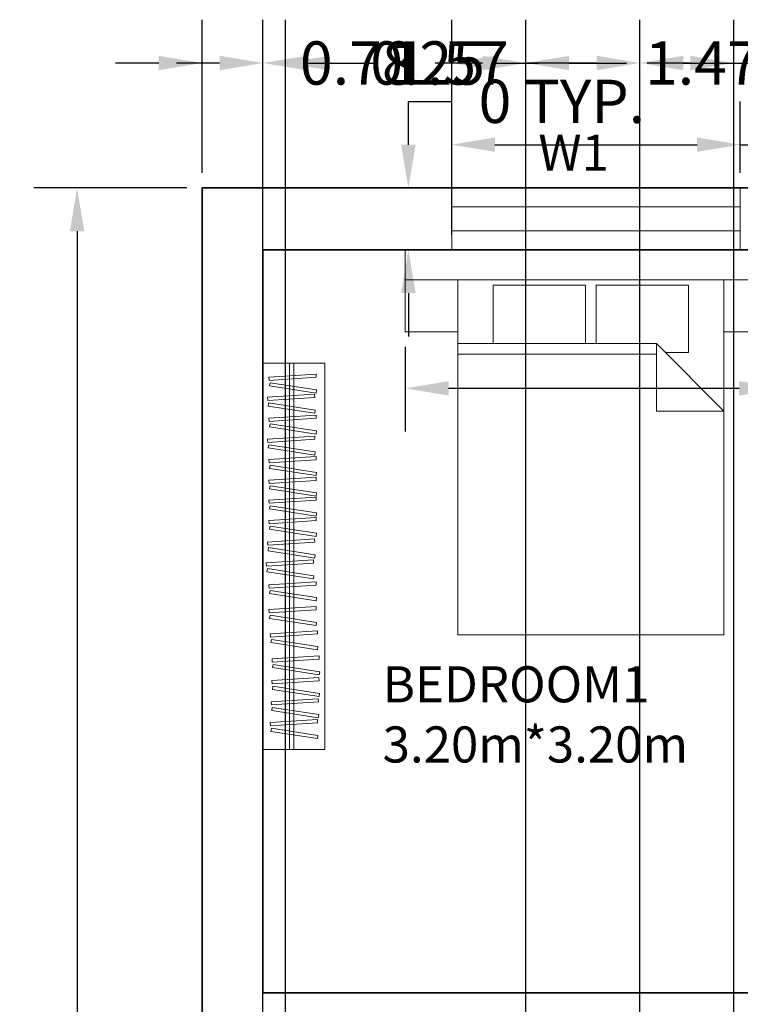
# Model space of a CAD drawing. Units: metres. Extents: x 1988.6 to 2001.1, y 2192 to 2202.5.
# Tile 3 of 6: x 1988.6 to 1991.6, y 2198.4 to 2202.5. Entities that reach past the tile are written whole.
import ezdxf

# ---------------------------------------------------------------- set-up
doc = ezdxf.new("R2010")
doc.units = ezdxf.units.M
for name, color, linetype, lineweight in [('A-ANNO-DIMS', 2, 'Continuous', 18), ('A-ANNO-TEXT', 7, 'Continuous', 18), ('A-AREA-IDEN', 7, 'Continuous', 18), ('A-FURN', 9, 'Continuous', 15), ('A-GLAZ', 4, 'Continuous', 18), ('A-WALL', 7, 'Continuous', 35)]:
    doc.layers.add(name, color=color, linetype=linetype, lineweight=lineweight)
doc.styles.get("Standard").update_dxf_attribs({"font": 'arial.ttf'})
doc.dimstyles.get("Standard").update_dxf_attribs({"dimtxt": 0.18, "dimasz": 0.18, "dimexe": 0.18, "dimexo": 0.0625, "dimgap": 0.09, "dimtad": 0, "dimtih": 1, "dimtoh": 1, "dimdec": 4, "dimzin": 0, "dimdsep": 46, "dimtxsty": 'Standard', "dimcen": 0.09, "dimadec": 0, "dimazin": 0, "dimtfac": 1, "dimtdec": 4, "dimtofl": 0, "dimtmove": 0, "dimatfit": 3, "dimfxl": 1, "dimtolj": 1, "dimtzin": 0, "dimarcsym": 0})

# ---------------------------------------------------------------- blocks, each defined once
blk = doc.blocks.new('Bed - Queen')
for p, q in [((0, -80.00003), (0, 0)), ((0, 0), (59.99999, 0)), ((59.99999, 0), (59.99999, -80.00003)), ((7.99999, -1.2), (28.79998, -1.2)), ((7.99999, -14.4), (7.99999, -1.2)), ((28.79998, -1.2), (28.79998, -14.4)), ((31.19999, -1.2), (51.99999, -1.2)), ((31.19999, -14.4), (31.19999, -1.2)), ((51.99999, -1.2), (51.99999, -16.4)), ((0, -14.4), (44.8, -14.4)), ((59.99999, -29.6), (44.8, -14.4)), ((44.8, -14.4), (44.8, -29.6)), ((44.8, -16.8), (0, -16.8)), ((51.99999, -16.4), (46.79936, -16.4)), ((44.8, -29.6), (59.99999, -29.6)), ((59.99999, -80.00003), (0, -80.00003))]:
    blk.add_line(p, q)
blk = doc.blocks.new('WIN-1200')
for p, q in [((-0.0002, 0.2568), (1.1998, 0.2568)), ((-0.0002, -0.0002), (-0.0002, 0.2568)), ((1.1998, 0.2568), (1.1998, -0.0002)), ((-0.0002, 0.1786), (1.1998, 0.1786)), ((-0.0002, 0.0793), (1.1998, 0.0793)), ((-0.0002, -0.0002), (1.1998, -0.0002))]:
    blk.add_line(p, q)
blk = doc.blocks.new('HEADBOARD-WITH-SIDE-TABLES')
for p, q in [((-0.0002, 0.3408), (-0.0002, 0.2164)), ((1.5674, 0.2164), (1.5674, 0.3408)), ((-0.0002, 0.2164), (1.5674, 0.2164)), ((-0.0002, 0.2164), (-0.0002, 0.0002)), ((1.5674, 0.2164), (1.5674, 0.0002)), ((-0.0002, 0.0002), (0.2181, 0.0002)), ((1.5674, 0.0002), (1.3249, 0.0002))]:
    blk.add_line(p, q)
blk = doc.blocks.new('WARDROBE-HANGING')
for p, q in [((0.0001, 1.6061), (0.2571, 1.6061)), ((0.0001, 1.6061), (0.0001, 0.0002)), ((0.1103, 1.6061), (0.1103, 0.0002)), ((0.1286, 1.6061), (0.1286, 0.0002)), ((0.2571, 1.6061), (0.2571, 0.0002)), ((0.2571, 0.0002), (0.0001, 0.0002))]:
    blk.add_line(p, q)
for points in [[(0.0252, 1.5475), (0.2208, 1.5602), (0.2217, 1.5468), (0.0261, 1.5341)], [(0.0296, 1.5242), (0.2233, 1.4943), (0.2212, 1.481), (0.0275, 1.5109)], [(0.0193, 1.4638), (0.2148, 1.4765), (0.2157, 1.4631), (0.0201, 1.4504)], [(0.0236, 1.4404), (0.2173, 1.4105), (0.2153, 1.3972), (0.0216, 1.4272)], [(0.0252, 1.377), (0.2208, 1.3897), (0.2217, 1.3763), (0.0261, 1.3636)], [(0.0296, 1.3537), (0.2233, 1.3238), (0.2212, 1.3105), (0.0275, 1.3404)], [(0.0196, 1.2897), (0.2152, 1.3024), (0.2161, 1.289), (0.0205, 1.2763)], [(0.024, 1.2664), (0.2177, 1.2365), (0.2157, 1.2232), (0.022, 1.2531)], [(0.0252, 1.205), (0.2208, 1.2177), (0.2217, 1.2043), (0.0261, 1.1916)], [(0.0296, 1.1817), (0.2233, 1.1517), (0.2212, 1.1385), (0.0275, 1.1684)], [(0.0252, 1.1192), (0.2208, 1.1319), (0.2217, 1.1185), (0.0261, 1.1058)], [(0.0296, 1.0959), (0.2233, 1.066), (0.2212, 1.0527), (0.0275, 1.0827)], [(0.0252, 1.0365), (0.2208, 1.0492), (0.2217, 1.0358), (0.0261, 1.0231)], [(0.0296, 1.0132), (0.2233, 0.9833), (0.2212, 0.97), (0.0275, 0.9999)], [(0.0252, 0.9518), (0.2208, 0.9645), (0.2217, 0.9511), (0.0261, 0.9384)], [(0.0296, 0.9285), (0.2233, 0.8986), (0.2212, 0.8853), (0.0275, 0.9152)], [(0.0193, 0.8621), (0.2148, 0.8748), (0.2157, 0.8614), (0.0201, 0.8487)], [(0.0236, 0.8388), (0.2173, 0.8089), (0.2153, 0.7956), (0.0216, 0.8255)], [(0.0141, 0.7752), (0.2097, 0.7879), (0.2106, 0.7745), (0.015, 0.7618)], [(0.0185, 0.7519), (0.2122, 0.722), (0.2101, 0.7087), (0.0164, 0.7386)], [(0.0252, 0.6841), (0.2208, 0.6968), (0.2217, 0.6834), (0.0261, 0.6707)], [(0.0296, 0.6608), (0.2233, 0.6309), (0.2212, 0.6176), (0.0275, 0.6475)], [(0.0252, 0.5812), (0.2208, 0.5939), (0.2217, 0.5805), (0.0261, 0.5678)], [(0.0296, 0.5578), (0.2233, 0.5279), (0.2212, 0.5146), (0.0275, 0.5446)], [(0.0307, 0.4806), (0.2263, 0.4933), (0.2272, 0.4799), (0.0316, 0.4672)], [(0.0351, 0.4573), (0.2288, 0.4273), (0.2268, 0.4141), (0.0331, 0.444)], [(0.0379, 0.3765), (0.2335, 0.3892), (0.2344, 0.3758), (0.0388, 0.3631)], [(0.0423, 0.3532), (0.236, 0.3232), (0.2339, 0.31), (0.0403, 0.3399)], [(0.0375, 0.286), (0.2331, 0.2987), (0.234, 0.2853), (0.0384, 0.2726)], [(0.0419, 0.2627), (0.2356, 0.2327), (0.2335, 0.2195), (0.0399, 0.2494)], [(0.0342, 0.1981), (0.2298, 0.2108), (0.2307, 0.1974), (0.0351, 0.1847)], [(0.0386, 0.1748), (0.2323, 0.1448), (0.2303, 0.1316), (0.0366, 0.1615)], [(0.0307, 0.1115), (0.2263, 0.1242), (0.2272, 0.1108), (0.0316, 0.0981)], [(0.0351, 0.0882), (0.2288, 0.0583), (0.2268, 0.045), (0.0331, 0.0749)]]:
    blk.add_lwpolyline(points, close=True)
blk = doc.blocks.new('*D32')
at = {"layer": 'A-ANNO-DIMS', "color": 0, "lineweight": -2, "transparency": 16777216}
for p, q in [((1990.4198, 2201.8163), (1990.4198, 2202.1138)), ((1991.6198, 2201.8163), (1991.6198, 2202.1138)), ((1990.5998, 2201.9338), (1991.4398, 2201.9338)), ((1991.6198, 2201.9338), (1991.7998, 2201.9338))]:
    blk.add_line(p, q, dxfattribs=at)
at = {"layer": 'A-ANNO-DIMS', "color": 0, "transparency": 16777216}
for points in [[(1990.5998, 2201.9638), (1990.5998, 2201.9038), (1990.4198, 2201.9338)], [(1991.4398, 2201.9638), (1991.4398, 2201.9038), (1991.6198, 2201.9338)]]:
    blk.add_solid(points, dxfattribs=at)
at = {"layer": 'Defpoints', "color": 0, "transparency": 16777216}
for p in [(1991.6198, 2201.9338), (1990.4198, 2201.7538), (1991.6198, 2201.7538)]:
    blk.add_point(p, dxfattribs=at)
at = {"layer": 'A-ANNO-DIMS', "color": 0, "transparency": 16777216, "insert": (1992.8625, 2201.9338), "char_height": 0.18, "attachment_point": 5}
blk.add_mtext('\\A1;WIN-1200 1 TYP.', dxfattribs=at)
blk = doc.blocks.new('*D33')
at = {"layer": 'A-ANNO-DIMS', "color": 0, "lineweight": -2, "transparency": 16777216}
for p, q in [((1990.2398, 2201.9338), (1990.2398, 2202.1138)), ((1990.2398, 2202.1138), (1990.4198, 2202.1138)), ((1990.3573, 2201.7538), (1990.0598, 2201.7538)), ((1990.3573, 2201.4968), (1990.0598, 2201.4968)), ((1990.2398, 2201.3168), (1990.2398, 2201.1368))]:
    blk.add_line(p, q, dxfattribs=at)
at = {"layer": 'A-ANNO-DIMS', "color": 0, "transparency": 16777216}
for points in [[(1990.2098, 2201.9338), (1990.2698, 2201.9338), (1990.2398, 2201.7538)], [(1990.2098, 2201.3168), (1990.2698, 2201.3168), (1990.2398, 2201.4968)]]:
    blk.add_solid(points, dxfattribs=at)
at = {"layer": 'Defpoints', "color": 0, "transparency": 16777216}
for p in [(1990.2398, 2201.7538), (1990.4198, 2201.7538), (1990.4198, 2201.4968)]:
    blk.add_point(p, dxfattribs=at)
at = {"layer": 'A-ANNO-DIMS', "color": 0, "transparency": 16777216, "insert": (1990.8779, 2202.1138), "char_height": 0.18, "attachment_point": 5}
blk.add_mtext('\\A1;0 TYP.', dxfattribs=at)
blk = doc.blocks.new('*D36')
at = {"layer": 'A-ANNO-DIMS', "color": 0, "lineweight": -2, "transparency": 16777216}
for p, q in [((1990.2268, 2201.0937), (1990.2268, 2200.741)), ((1991.7944, 2201.0937), (1991.7944, 2200.741)), ((1990.4068, 2200.921), (1991.6144, 2200.921)), ((1991.7944, 2200.921), (1991.9744, 2200.921))]:
    blk.add_line(p, q, dxfattribs=at)
at = {"layer": 'A-ANNO-DIMS', "color": 0, "transparency": 16777216}
for points in [[(1990.4068, 2200.951), (1990.4068, 2200.891), (1990.2268, 2200.921)], [(1991.6144, 2200.951), (1991.6144, 2200.891), (1991.7944, 2200.921)]]:
    blk.add_solid(points, dxfattribs=at)
at = {"layer": 'Defpoints', "color": 0, "transparency": 16777216}
for p in [(1990.2268, 2201.1562), (1991.7944, 2201.1562), (1991.7944, 2200.921)]:
    blk.add_point(p, dxfattribs=at)
at = {"layer": 'A-ANNO-DIMS', "color": 0, "transparency": 16777216, "insert": (1993.5874, 2200.921), "char_height": 0.18, "attachment_point": 5}
blk.add_mtext('\\A1;HEADBOARD UNIT 2 TYP.', dxfattribs=at)
blk = doc.blocks.new('*D53')
at = {"layer": 'A-ANNO-DIMS', "color": 0, "lineweight": -2, "transparency": 16777216}
for p, q in [((1989.3193, 2201.7538), (1988.6823, 2201.7538)), ((1988.8623, 2201.5738), (1988.8623, 2197.4107)), ((1988.8623, 2192.8838), (1988.8623, 2197.0469)), ((1989.3193, 2192.7038), (1988.6823, 2192.7038))]:
    blk.add_line(p, q, dxfattribs=at)
at = {"layer": 'A-ANNO-DIMS', "color": 0, "transparency": 16777216}
for points in [[(1988.8323, 2201.5738), (1988.8923, 2201.5738), (1988.8623, 2201.7538)], [(1988.8323, 2192.8838), (1988.8923, 2192.8838), (1988.8623, 2192.7038)]]:
    blk.add_solid(points, dxfattribs=at)
at = {"layer": 'Defpoints', "color": 0, "transparency": 16777216}
for p in [(1988.8623, 2201.7538), (1989.3818, 2201.7538), (1989.3818, 2192.7038)]:
    blk.add_point(p, dxfattribs=at)
at = {"layer": 'A-ANNO-DIMS', "color": 0, "transparency": 16777216, "insert": (1988.8623, 2197.2288), "char_height": 0.18, "attachment_point": 5}
blk.add_mtext('\\A1;9.05', dxfattribs=at)
blk = doc.blocks.new('*D54')
at = {"layer": 'A-ANNO-DIMS', "color": 0, "lineweight": -2, "transparency": 16777216}
for p, q in [((1989.6351, 2201.5593), (1989.6351, 2202.4533)), ((1990.4198, 2201.5593), (1990.4198, 2202.4533)), ((1989.4551, 2202.2733), (1989.2751, 2202.2733)), ((1990.5998, 2202.2733), (1990.7798, 2202.2733))]:
    blk.add_line(p, q, dxfattribs=at)
at = {"layer": 'A-ANNO-DIMS', "color": 0, "transparency": 16777216}
for points in [[(1989.4551, 2202.3033), (1989.4551, 2202.2433), (1989.6351, 2202.2733)], [(1990.5998, 2202.3033), (1990.5998, 2202.2433), (1990.4198, 2202.2733)]]:
    blk.add_solid(points, dxfattribs=at)
at = {"layer": 'Defpoints', "color": 0, "transparency": 16777216}
for p in [(1990.4198, 2202.2733), (1989.6351, 2201.4968), (1990.4198, 2201.4968)]:
    blk.add_point(p, dxfattribs=at)
at = {"layer": 'A-ANNO-DIMS', "color": 0, "transparency": 16777216, "insert": (1990.0275, 2202.2733), "char_height": 0.18, "attachment_point": 5}
blk.add_mtext('\\A1;0.78', dxfattribs=at)
blk = doc.blocks.new('*D59')
at = {"layer": 'A-ANNO-DIMS', "color": 0, "lineweight": -2, "transparency": 16777216}
for p, q in [((1989.7282, 2194.023), (1989.7282, 2202.4533)), ((1990.7282, 2193.0163), (1990.7282, 2202.4533)), ((1989.9082, 2202.2733), (1990.1051, 2202.2733)), ((1990.5482, 2202.2733), (1990.3514, 2202.2733))]:
    blk.add_line(p, q, dxfattribs=at)
at = {"layer": 'A-ANNO-DIMS', "color": 0, "transparency": 16777216}
for points in [[(1989.9082, 2202.3033), (1989.9082, 2202.2433), (1989.7282, 2202.2733)], [(1990.5482, 2202.3033), (1990.5482, 2202.2433), (1990.7282, 2202.2733)]]:
    blk.add_solid(points, dxfattribs=at)
at = {"layer": 'Defpoints', "color": 0, "transparency": 16777216}
for p in [(1990.7282, 2202.2733), (1989.7282, 2193.9605), (1990.7282, 2192.9538)]:
    blk.add_point(p, dxfattribs=at)
at = {"layer": 'A-ANNO-DIMS', "color": 0, "transparency": 16777216, "insert": (1990.2282, 2202.2733), "char_height": 0.18, "attachment_point": 5}
blk.add_mtext('\\A1;1', dxfattribs=at)
blk = doc.blocks.new('*D60')
at = {"layer": 'A-ANNO-DIMS', "color": 0, "lineweight": -2, "transparency": 16777216}
for p, q in [((1990.7282, 2193.0163), (1990.7282, 2202.4533)), ((1992.1958, 2193.0163), (1992.1958, 2202.4533)), ((1990.9082, 2202.2733), (1991.1467, 2202.2733)), ((1992.0158, 2202.2733), (1991.7773, 2202.2733))]:
    blk.add_line(p, q, dxfattribs=at)
at = {"layer": 'A-ANNO-DIMS', "color": 0, "transparency": 16777216}
for points in [[(1990.9082, 2202.3033), (1990.9082, 2202.2433), (1990.7282, 2202.2733)], [(1992.0158, 2202.3033), (1992.0158, 2202.2433), (1992.1958, 2202.2733)]]:
    blk.add_solid(points, dxfattribs=at)
at = {"layer": 'Defpoints', "color": 0, "transparency": 16777216}
for p in [(1992.1958, 2202.2733), (1990.7282, 2192.9538), (1992.1958, 2192.9538)]:
    blk.add_point(p, dxfattribs=at)
at = {"layer": 'A-ANNO-DIMS', "color": 0, "transparency": 16777216, "insert": (1991.462, 2202.2733), "char_height": 0.18, "attachment_point": 5}
blk.add_mtext('\\A1;1.47', dxfattribs=at)
blk = doc.blocks.new('*D62')
at = {"layer": 'A-ANNO-DIMS', "color": 0, "lineweight": -2, "transparency": 16777216}
for p, q in [((1989.6351, 2193.0163), (1989.6351, 2202.4533)), ((1991.2026, 2195.283), (1991.2026, 2202.4533)), ((1989.8151, 2202.2733), (1990.1035, 2202.2733)), ((1991.0226, 2202.2733), (1990.7342, 2202.2733))]:
    blk.add_line(p, q, dxfattribs=at)
at = {"layer": 'A-ANNO-DIMS', "color": 0, "transparency": 16777216}
for points in [[(1989.8151, 2202.3033), (1989.8151, 2202.2433), (1989.6351, 2202.2733)], [(1991.0226, 2202.3033), (1991.0226, 2202.2433), (1991.2026, 2202.2733)]]:
    blk.add_solid(points, dxfattribs=at)
at = {"layer": 'Defpoints', "color": 0, "transparency": 16777216}
for p in [(1991.2026, 2202.2733), (1991.2026, 2195.2205), (1989.6351, 2192.9538)]:
    blk.add_point(p, dxfattribs=at)
at = {"layer": 'A-ANNO-DIMS', "color": 0, "transparency": 16777216, "insert": (1990.4189, 2202.2733), "char_height": 0.18, "attachment_point": 5}
blk.add_mtext('\\A1;1.57', dxfattribs=at)
blk = doc.blocks.new('*D63')
at = {"layer": 'A-ANNO-DIMS', "color": 0, "lineweight": -2, "transparency": 16777216}
for p, q in [((1991.2026, 2195.283), (1991.2026, 2202.4533)), ((1995.1007, 2195.283), (1995.1007, 2202.4533)), ((1991.3826, 2202.2733), (1992.7578, 2202.2733)), ((1994.9207, 2202.2733), (1993.5455, 2202.2733))]:
    blk.add_line(p, q, dxfattribs=at)
at = {"layer": 'A-ANNO-DIMS', "color": 0, "transparency": 16777216}
for points in [[(1991.3826, 2202.3033), (1991.3826, 2202.2433), (1991.2026, 2202.2733)], [(1994.9207, 2202.3033), (1994.9207, 2202.2433), (1995.1007, 2202.2733)]]:
    blk.add_solid(points, dxfattribs=at)
at = {"layer": 'Defpoints', "color": 0, "transparency": 16777216}
for p in [(1995.1007, 2202.2733), (1991.2026, 2195.2205), (1995.1007, 2195.2205)]:
    blk.add_point(p, dxfattribs=at)
at = {"layer": 'A-ANNO-DIMS', "color": 0, "transparency": 16777216, "insert": (1993.1516, 2202.2733), "char_height": 0.18, "attachment_point": 5}
blk.add_mtext('\\A1;3.898', dxfattribs=at)
blk = doc.blocks.new('*D67')
at = {"layer": 'A-ANNO-DIMS', "color": 0, "lineweight": -2, "transparency": 16777216}
for p, q in [((1991.5924, 2194.3163), (1991.5924, 2202.4533)), ((1991.9822, 2194.3163), (1991.9822, 2202.4533)), ((1991.4124, 2202.2733), (1991.2324, 2202.2733)), ((1992.1622, 2202.2733), (1992.3422, 2202.2733))]:
    blk.add_line(p, q, dxfattribs=at)
at = {"layer": 'A-ANNO-DIMS', "color": 0, "transparency": 16777216}
for points in [[(1991.4124, 2202.3033), (1991.4124, 2202.2433), (1991.5924, 2202.2733)], [(1992.1622, 2202.3033), (1992.1622, 2202.2433), (1991.9822, 2202.2733)]]:
    blk.add_solid(points, dxfattribs=at)
at = {"layer": 'Defpoints', "color": 0, "transparency": 16777216}
for p in [(1991.9822, 2202.2733), (1991.5924, 2194.2538), (1991.9822, 2194.2538)]:
    blk.add_point(p, dxfattribs=at)
at = {"layer": 'A-ANNO-DIMS', "color": 0, "transparency": 16777216, "insert": (1992.6662, 2202.2733), "char_height": 0.18, "attachment_point": 5}
blk.add_mtext('\\A1;0.39', dxfattribs=at)
blk = doc.blocks.new('*D76')
at = {"layer": 'A-ANNO-DIMS', "color": 0, "lineweight": -2, "transparency": 16777216}
for p, q in [((1989.3818, 2201.8163), (1989.3818, 2202.4533)), ((1989.6351, 2201.5593), (1989.6351, 2202.4533)), ((1989.2018, 2202.2733), (1989.0218, 2202.2733)), ((1989.8151, 2202.2733), (1989.9951, 2202.2733))]:
    blk.add_line(p, q, dxfattribs=at)
at = {"layer": 'A-ANNO-DIMS', "color": 0, "transparency": 16777216}
for points in [[(1989.2018, 2202.3033), (1989.2018, 2202.2433), (1989.3818, 2202.2733)], [(1989.8151, 2202.3033), (1989.8151, 2202.2433), (1989.6351, 2202.2733)]]:
    blk.add_solid(points, dxfattribs=at)
at = {"layer": 'Defpoints', "color": 0, "transparency": 16777216}
for p in [(1989.6351, 2202.2733), (1989.3818, 2201.7538), (1989.6351, 2201.4968)]:
    blk.add_point(p, dxfattribs=at)
at = {"layer": 'A-ANNO-DIMS', "color": 0, "transparency": 16777216, "insert": (1990.3196, 2202.2733), "char_height": 0.18, "attachment_point": 5}
blk.add_mtext('\\A1;0.25', dxfattribs=at)

msp = doc.modelspace()

# ---------------------------------------------------------------- linework, layer by layer
at = {"layer": 'A-WALL'}
for p, q in [((1989.3818, 2201.7538), (1989.3818, 2192.7038)), ((1999.3818, 2201.7538), (1989.3818, 2201.7538)), ((1989.6351, 2201.4968), (1989.6351, 2198.4088)), ((1992.6858, 2201.4968), (1989.6351, 2201.4968)), ((1992.6858, 2198.4088), (1989.6351, 2198.4088))]:
    msp.add_line(p, q, dxfattribs=at)

# ---------------------------------------------------------------- block references
at = {"layer": 'A-FURN'}
for name, p in [('HEADBOARD-WITH-SIDE-TABLES', (1990.227, 2201.156)), ('WARDROBE-HANGING', (1989.635, 2199.42))]:
    msp.add_blockref(name, p, dxfattribs=at)
at = {"layer": 'A-FURN', "xscale": 0.0184456424226754, "yscale": 0.0184456424226754, "zscale": 0.0184456424226754}
msp.add_blockref('Bed - Queen', (1990.4451, 2201.3724), dxfattribs=at)
at = {"layer": 'A-GLAZ'}
msp.add_blockref('WIN-1200', (1990.42, 2201.497), dxfattribs=at)

# ---------------------------------------------------------------- texts
at = {"layer": 'A-ANNO-TEXT', "insert": (1990.7801, 2201.9754), "char_height": 0.15, "attachment_point": 1}
msp.add_mtext_dynamic_manual_height_columns('W1', width=0.386628, gutter_width=12.5, heights=[0], dxfattribs=at)
at = {"layer": 'A-AREA-IDEN', "insert": (1990.1328, 2199.7657), "char_height": 0.15, "attachment_point": 1}
msp.add_mtext_dynamic_manual_height_columns('BEDROOM1 3.20m*3.20m', width=1.796061, gutter_width=12.5, heights=[0], dxfattribs=at)

# ---------------------------------------------------------------- dimensions: what is measured, and where the dimension line sits
at = {"layer": 'A-ANNO-DIMS'}
for base, p1, p2, override, picture, middle in [((1989.6351, 2202.2733), (1989.3818, 2201.7538), (1989.6351, 2201.4968), {"dimdec": 2, "dimlfac": 1, "dimrnd": 0, "dimzin": 0, "dimdsep": 46, "dimlunit": 2}, '*D76', (1990.3196, 2202.2733)), ((1990.4198, 2202.2733), (1989.6351, 2201.4968), (1990.4198, 2201.4968), {"dimdec": 2, "dimlfac": 1, "dimrnd": 0, "dimzin": 0, "dimdsep": 46, "dimlunit": 2}, '*D54', (1990.0275, 2202.2733)), ((1991.2026, 2202.2733), (1989.6351, 2192.9538), (1991.2026, 2195.2205), {"dimdec": 2, "dimlfac": 1, "dimrnd": 0, "dimzin": 0, "dimdsep": 46, "dimlunit": 2}, '*D62', (1990.4189, 2202.2733)), ((1990.7282, 2202.2733), (1989.7282, 2193.9605), (1990.7282, 2192.9538), {"dimdec": 0, "dimlfac": 1, "dimrnd": 0, "dimzin": 0, "dimdsep": 46, "dimlunit": 2}, '*D59', (1990.2282, 2202.2733)), ((1992.1958, 2202.2733), (1990.7282, 2192.9538), (1992.1958, 2192.9538), {"dimdec": 2, "dimlfac": 1, "dimrnd": 0, "dimzin": 0, "dimdsep": 46, "dimlunit": 2}, '*D60', (1991.462, 2202.2733)), ((1995.1007, 2202.2733), (1991.2026, 2195.2205), (1995.1007, 2195.2205), {"dimdec": 3, "dimlfac": 1, "dimrnd": 0, "dimzin": 0, "dimdsep": 46, "dimlunit": 2}, '*D63', (1993.1516, 2202.2733)), ((1991.9822, 2202.2733), (1991.5924, 2194.2538), (1991.9822, 2194.2538), {"dimdec": 2, "dimlfac": 1, "dimrnd": 0, "dimzin": 0, "dimdsep": 46, "dimlunit": 2}, '*D67', (1992.6662, 2202.2733))]:
    dim = msp.add_linear_dim(base=base, p1=p1, p2=p2, dimstyle='Standard', override=override, dxfattribs=at)
    dim.commit()
    dim.dimension.update_dxf_attribs({"geometry": picture, "text_midpoint": middle})
dim = msp.add_linear_dim(base=(1990.2398, 2201.7538), p1=(1990.4198, 2201.4968), p2=(1990.4198, 2201.7538), angle=90, text='<> TYP.', dimstyle='Standard', override={"dimdec": 0, "dimlfac": 1, "dimrnd": 0, "dimzin": 0, "dimdsep": 46, "dimlunit": 2}, dxfattribs=at)
dim.commit()
dim.dimension.update_dxf_attribs({"geometry": '*D33', "text_midpoint": (1990.8779, 2202.1138)})
for base, p1, p2, text, picture, middle in [((1991.6198, 2201.9338), (1990.4198, 2201.7538), (1991.6198, 2201.7538), 'WIN-1200 <> TYP.', '*D32', (1992.8625, 2201.9338)), ((1991.7944, 2200.921), (1990.2268, 2201.1562), (1991.7944, 2201.1562), 'HEADBOARD UNIT <> TYP.', '*D36', (1993.5874, 2200.921))]:
    dim = msp.add_linear_dim(base=base, p1=p1, p2=p2, text=text, dimstyle='Standard', override={"dimdec": 0, "dimlfac": 1, "dimrnd": 0, "dimzin": 0, "dimdsep": 46, "dimlunit": 2}, dxfattribs=at)
    dim.commit()
    dim.dimension.update_dxf_attribs({"geometry": picture, "text_midpoint": middle})
dim = msp.add_linear_dim(base=(1988.8623, 2201.7538), p1=(1989.3818, 2192.7038), p2=(1989.3818, 2201.7538), angle=90, dimstyle='Standard', override={"dimdec": 2, "dimlfac": 1, "dimrnd": 0, "dimzin": 0, "dimdsep": 46, "dimlunit": 2}, dxfattribs=at)
dim.commit()
dim.dimension.update_dxf_attribs({"geometry": '*D53', "text_midpoint": (1988.8623, 2197.2288)})

doc.saveas('drawing.dxf')
